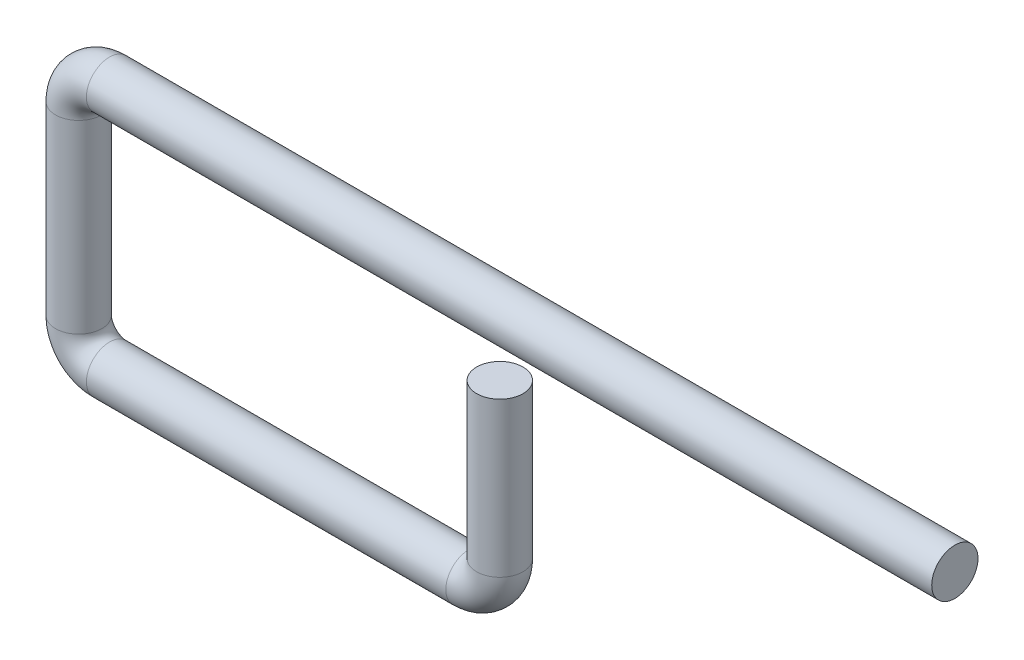
SolidWorks part; units mm, degrees
material "Plain Carbon Steel"
ref_plane "Front Plane" through (0, 0, 0) normal (0, 0, 1) x (1, 0, 0)
ref_plane "Top Plane" through (0, 0, 0) normal (0, 1, 0) x (1, 0, 0)
ref_plane "Right Plane" through (0, 0, 0) normal (1, 0, 0) x (0, 0, -1)
sketch "Bolt Rod Path" plane through (0, 0, 0) normal (0, 0, 1) x (1, 0, 0)
  line L0 (0, 0) -> (0, -25)
  line L1 (-5, -30) -> (-63.25, -30)
  line L2 (-68.25, -25) -> (-68.25, 5)
  line L3 (-63.25, 10) -> (73.75, 10)
  arc A0 (0, -25) -> (-5, -30) centre (-5, -25) cw
  arc A1 (-63.25, -30) -> (-68.25, -25) centre (-63.25, -25) cw
  arc A2 (-68.25, 5) -> (-63.25, 10) centre (-63.25, 5) cw
  point P8 (0, -30)
  point P11 (-68.25, -30)
  point P14 (-68.25, 10)
  dimension "D5" = 5
  dimension "D1" = 142
  dimension "D2" = 68.25
  dimension "D3" = 40
  dimension "D4" = 30
sweep "Bolt Rod Sweep Ø7.5" add path "Bolt Rod Path" circular profile diameter 7.5 parameters "D3"=7.5
